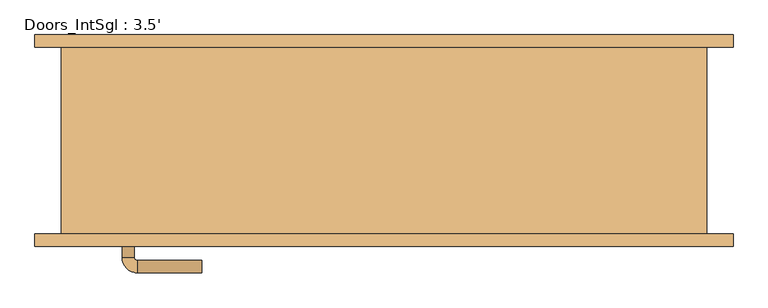
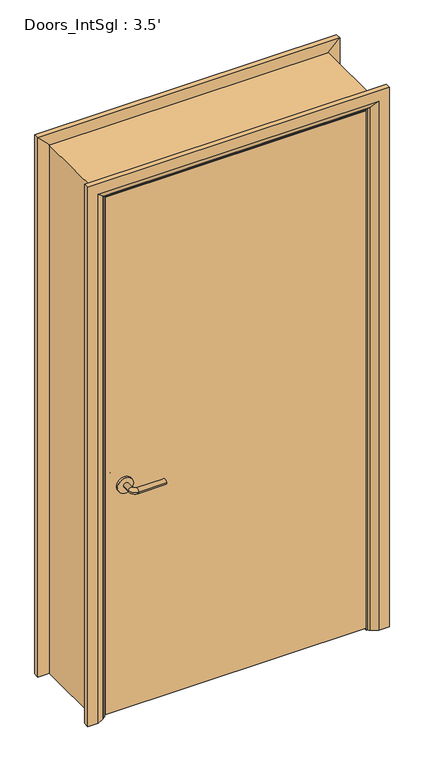
"""IFC4 building model written with IfcOpenShell, lengths in millimetres: door geometry, Doors_IntSgl : 3.5'."""

from ifc_helpers import new_model, si_unit, point, frame, frame_2d, origin, place, context, project, spatial, polyline, circle_curve, ellipse_curve, trimmed, segment, composite_curve, outline, extrude, faceted_brep, source, transform, mapped, element, save
from ifc_brep_helpers import plane_surface, cylinder_surface, revolved_surface, advanced_brep


def doors_intsgl_3_5_f2e8c556(model_context):
    return source(origin(), model_context, "Body", "SolidModel", [
        advanced_brep(
        [(-426.4, -106.4, 900.0), (-406.4, -106.4, 900.0), (-426.4, -76.4, 900.0), (-406.4, -76.4, 900.0), (-401.4, -71.4, 900.0), (-401.4, -51.4, 900.0), (-296.4, -51.4, 900.0), (-296.4, -71.4, 900.0)],
        [
            (0, 1, circle_curve(frame((-416.4, -106.4, 900.0), z_axis=(0.0, -1.0, 0.0), x_axis=(1.0, 0.0, 0.0)), 10.0)),
            (1, 0, circle_curve(frame((-416.4, -106.4, 900.0), z_axis=(0.0, -1.0, 0.0), x_axis=(1.0, 0.0, 0.0)), 10.0)),
            (0, 2),
            (2, 3, circle_curve(frame((-416.4, -76.4, 900.0), z_axis=(0.0, -1.0, 0.0), x_axis=(1.0, 0.0, 0.0)), 10.0)),
            (3, 1),
            (3, 2, circle_curve(frame((-416.4, -76.4, 900.0), z_axis=(0.0, -1.0, 0.0), x_axis=(1.0, 0.0, 0.0)), 10.0)),
            (4, 3, circle_curve(frame((-401.4, -76.4, 900.0), z_axis=(0.0, 0.0, 1.0), x_axis=(-1.0, 0.0, 0.0)), 5.0)),
            (2, 5, circle_curve(frame((-401.4, -76.4, 900.0), z_axis=(0.0, 0.0, -1.0), x_axis=(-1.0, 0.0, 0.0)), 25.0)),
            (5, 4, circle_curve(frame((-401.4, -61.4, 900.0), z_axis=(-1.0, 0.0, 0.0), x_axis=(0.0, -1.0, 0.0)), 10.0)),
            (4, 5, circle_curve(frame((-401.4, -61.4, 900.0), z_axis=(-1.0, 0.0, 0.0), x_axis=(0.0, -1.0, 0.0)), 10.0)),
            (6, 7, circle_curve(frame((-296.4, -61.4, 900.0), z_axis=(1.0, 0.0, 0.0), x_axis=(0.0, -1.0, 0.0)), 10.0)),
            (7, 6, circle_curve(frame((-296.4, -61.4, 900.0), z_axis=(1.0, 0.0, 0.0), x_axis=(0.0, -1.0, 0.0)), 10.0)),
            (5, 6),
            (7, 4),
        ],
        [
            plane_surface(frame((-416.4, -106.4, 900.0), z_axis=(0.0, -1.0, 0.0), x_axis=(0.0, 0.0, 1.0))),
            cylinder_surface(frame((-416.4, -106.4, 900.0), z_axis=(0.0, -1.0, 0.0), x_axis=(1.0, 0.0, 0.0)), 10.0),
            revolved_surface(trimmed(ellipse_curve(frame((-416.4, -76.4, 900.0), z_axis=(0.0, -1.0, 0.0), x_axis=(1.0, 0.0, 0.0)), 10.0, 10.0), [point((-426.4, -76.4, 900.0))], [point((-406.4, -76.4, 900.0))], True, "CARTESIAN"), (-401.4, -76.4, 900.0), (0.0, 0.0, -1.0)),
            revolved_surface(trimmed(ellipse_curve(frame((-416.4, -76.4, 900.0), z_axis=(0.0, -1.0, 0.0), x_axis=(1.0, 0.0, 0.0)), 10.0, 10.0), [point((-406.4, -76.4, 900.0))], [point((-426.4, -76.4, 900.0))], True, "CARTESIAN"), (-401.4, -76.4, 900.0), (0.0, 0.0, -1.0)),
            plane_surface(frame((-296.4, -61.4, 900.0), z_axis=(1.0, 0.0, 0.0), x_axis=(0.0, 0.0, 1.0))),
            cylinder_surface(frame((-401.4, -61.4, 900.0), z_axis=(-1.0, 0.0, 0.0), x_axis=(0.0, -1.0, 0.0)), 10.0),
        ],
        [
            (0, [[1, 2]]),
            (1, [[-1, 3, 4, 5]]),
            (1, [[-2, -5, 6, -3]]),
            (2, [[7, -4, 8, 9]]),
            (3, [[-8, -6, -7, 10]]),
            (4, [[11, 12]]),
            (5, [[-9, 13, -12, 14]]),
            (5, [[-10, -14, -11, -13]]),
        ],
    ),
        extrude(outline(composite_curve([segment(trimmed(circle_curve(frame_2d((900.0, -418.9)), 30.0), [point((900.0, -448.9))], [point((900.0, -388.9))], False, "CARTESIAN"), True, "CONTINUOUS"), segment(trimmed(circle_curve(frame_2d((900.0, -418.9)), 30.0), [point((900.0, -388.9))], [point((900.0, -448.9))], False, "CARTESIAN"), True, "CONTINUOUS")], self_intersect=False)), frame((0.0, -114.4, 0.0), z_axis=(0.0, 1.0, 0.0), x_axis=(0.0, 0.0, 1.0)), (0.0, 0.0, 1.0), 8.0),
        advanced_brep(
        [(-426.4, -160.4, 900.0), (-406.4, -160.4, 900.0), (-406.4, -190.4, 900.0), (-426.4, -190.4, 900.0), (-401.4, -195.4, 900.0), (-401.4, -215.4, 900.0), (-296.4, -215.4, 900.0), (-296.4, -195.4, 900.0)],
        [
            (0, 1, circle_curve(frame((-416.4, -160.4, 900.0), z_axis=(0.0, 1.0, 0.0), x_axis=(1.0, 0.0, 0.0)), 10.0)),
            (1, 0, circle_curve(frame((-416.4, -160.4, 900.0), z_axis=(0.0, 1.0, 0.0), x_axis=(1.0, 0.0, 0.0)), 10.0)),
            (1, 2),
            (2, 3, circle_curve(frame((-416.4, -190.4, 900.0), z_axis=(0.0, 1.0, 0.0), x_axis=(1.0, 0.0, 0.0)), 10.0)),
            (3, 0),
            (3, 2, circle_curve(frame((-416.4, -190.4, 900.0), z_axis=(0.0, 1.0, 0.0), x_axis=(1.0, 0.0, 0.0)), 10.0)),
            (4, 5, circle_curve(frame((-401.4, -205.4, 900.0), z_axis=(-1.0, 0.0, 0.0), x_axis=(0.0, 1.0, 0.0)), 10.0)),
            (5, 3, circle_curve(frame((-401.4, -190.4, 900.0), z_axis=(0.0, 0.0, -1.0), x_axis=(-1.0, 0.0, 0.0)), 25.0)),
            (2, 4, circle_curve(frame((-401.4, -190.4, 900.0), z_axis=(0.0, 0.0, 1.0), x_axis=(-1.0, 0.0, 0.0)), 5.0)),
            (5, 4, circle_curve(frame((-401.4, -205.4, 900.0), z_axis=(-1.0, 0.0, 0.0), x_axis=(0.0, 1.0, 0.0)), 10.0)),
            (6, 7, circle_curve(frame((-296.4, -205.4, 900.0), z_axis=(1.0, 0.0, 0.0), x_axis=(0.0, 1.0, 0.0)), 10.0)),
            (7, 6, circle_curve(frame((-296.4, -205.4, 900.0), z_axis=(1.0, 0.0, 0.0), x_axis=(0.0, 1.0, 0.0)), 10.0)),
            (4, 7),
            (6, 5),
        ],
        [
            plane_surface(frame((-416.4, -160.4, 900.0), z_axis=(0.0, 1.0, 0.0), x_axis=(0.0, 0.0, 1.0))),
            cylinder_surface(frame((-416.4, -160.4, 900.0), z_axis=(0.0, 1.0, 0.0), x_axis=(1.0, 0.0, 0.0)), 10.0),
            revolved_surface(trimmed(ellipse_curve(frame((-416.4, -190.4, 900.0), z_axis=(0.0, -1.0, 0.0), x_axis=(1.0, 0.0, 0.0)), 10.0, 10.0), [point((-426.4, -190.4, 900.0))], [point((-406.4, -190.4, 900.0))], True, "CARTESIAN"), (-401.4, -190.4, 900.0), (0.0, 0.0, -1.0)),
            revolved_surface(trimmed(ellipse_curve(frame((-416.4, -190.4, 900.0), z_axis=(0.0, -1.0, 0.0), x_axis=(1.0, 0.0, 0.0)), 10.0, 10.0), [point((-406.4, -190.4, 900.0))], [point((-426.4, -190.4, 900.0))], True, "CARTESIAN"), (-401.4, -190.4, 900.0), (0.0, 0.0, -1.0)),
            plane_surface(frame((-296.4, -205.4, 900.0), z_axis=(1.0, 0.0, 0.0), x_axis=(0.0, 0.0, 1.0))),
            cylinder_surface(frame((-401.4, -205.4, 900.0), z_axis=(-1.0, 0.0, 0.0), x_axis=(0.0, 1.0, 0.0)), 10.0),
        ],
        [
            (0, [[1, 2]]),
            (1, [[3, 4, 5, -2]]),
            (1, [[-5, 6, -3, -1]]),
            (2, [[7, 8, -4, 9]]),
            (3, [[10, -9, -6, -8]]),
            (4, [[11, 12]]),
            (5, [[13, -11, 14, -7]]),
            (5, [[-14, -12, -13, -10]]),
        ],
    ),
        extrude(outline(composite_curve([segment(trimmed(circle_curve(frame_2d((900.0, -418.9)), 30.0), [point((900.0, -448.9))], [point((900.0, -388.9))], False, "CARTESIAN"), True, "CONTINUOUS"), segment(trimmed(circle_curve(frame_2d((900.0, -418.9)), 30.0), [point((900.0, -388.9))], [point((900.0, -448.9))], False, "CARTESIAN"), True, "CONTINUOUS")], self_intersect=False)), frame((0.0, -160.4, 0.0), z_axis=(0.0, 1.0, 0.0), x_axis=(0.0, 0.0, 1.0)), (0.0, 0.0, 1.0), 8.0),
        extrude(outline(polyline([(491.4, -114.4), (491.4, -152.4), (-491.4, -152.4), (-491.4, -114.4), (491.4, -114.4)])), frame((0.0, 0.0, 8.0), z_axis=(0.0, 0.0, 1.0), x_axis=(1.0, 0.0, 0.0)), (0.0, 0.0, 1.0), 2060.0),
        advanced_brep(
        [(568.4, -172.4, 0.0), (528.4, -172.4, 0.0), (502.4, -158.4, 0.0), (498.4, -152.4, 0.0), (568.4, -152.4, 0.0), (568.4, -152.4, 2145.0), (568.4, -172.4, 2145.0), (498.4, -152.4, 2075.0), (-498.4, -152.4, 2075.0), (-498.4, -152.4, 0.0), (-568.4, -152.4, 0.0), (-568.4, -152.4, 2145.0), (502.4, -158.4, 2079.0), (528.4, -172.4, 2105.0), (-568.4, -172.4, 2145.0), (-568.4, -172.4, 0.0), (-528.4, -172.4, 0.0), (-528.4, -172.4, 2105.0), (-502.4, -158.4, 0.0), (-502.4, -158.4, 2079.0)],
        [
            (0, 1),
            (1, 2),
            (2, 3, circle_curve(frame((506.4, -151.4, 0.0), z_axis=(0.0, 0.0, -1.0), x_axis=(1.0, 0.0, 0.0)), 8.0622577)),
            (3, 4),
            (4, 0),
            (4, 5),
            (5, 6),
            (6, 0),
            (3, 7),
            (7, 8),
            (8, 9),
            (9, 10),
            (10, 11),
            (11, 5),
            (2, 12),
            (12, 7, ellipse_curve(frame((506.4, -151.4, 2083.0), z_axis=(0.7071067811865475, 0.0, -0.7071067811865475), x_axis=(-0.7071067811865474, 0.0, -0.7071067811865476)), 11.4017543, 8.0622577)),
            (1, 13),
            (13, 12),
            (6, 14),
            (14, 15),
            (15, 16),
            (16, 17),
            (17, 13),
            (10, 15),
            (14, 11),
            (9, 18, circle_curve(frame((-506.4, -151.4, 0.0), z_axis=(0.0, 0.0, -1.0), x_axis=(-1.0, 0.0, 0.0)), 8.0622577)),
            (18, 16),
            (19, 18),
            (8, 19, ellipse_curve(frame((-506.4, -151.4, 2083.0), z_axis=(-0.7071067811865475, 0.0, -0.7071067811865475), x_axis=(-0.7071067811865474, 0.0, 0.7071067811865476)), 11.4017543, 8.0622577)),
            (19, 17),
            (12, 19),
        ],
        [
            plane_surface(frame((498.4, -152.4, 0.0), z_axis=(0.0, 0.0, -1.0), x_axis=(0.0, 1.0, 0.0))),
            plane_surface(frame((568.4, -172.4, 0.0), z_axis=(1.0, 0.0, 0.0), x_axis=(0.0, 0.0, 1.0))),
            plane_surface(frame((568.4, -152.4, 0.0), z_axis=(0.0, 1.0, 0.0), x_axis=(0.0, 0.0, 1.0))),
            cylinder_surface(frame((506.4, -151.4, 0.0), z_axis=(0.0, 0.0, -1.0), x_axis=(1.0, 0.0, 0.0)), 8.0622577),
            plane_surface(frame((502.4, -158.4, 0.0), z_axis=(-0.4740998230350126, -0.880471099922178, 0.0), x_axis=(0.0, 0.0, 1.0))),
            plane_surface(frame((528.4, -172.4, 0.0), z_axis=(0.0, -1.0, 0.0), x_axis=(0.0, 0.0, 1.0))),
            plane_surface(frame((-568.4, -172.4, 2145.0), z_axis=(-1.0, 0.0, 0.0), x_axis=(0.0, 0.0, -1.0))),
            plane_surface(frame((-498.4, -152.4, 0.0), z_axis=(0.0, 0.0, -1.0), x_axis=(0.0, 1.0, 0.0))),
            cylinder_surface(frame((-506.4, -151.4, 2075.0), z_axis=(0.0, 0.0, 1.0), x_axis=(-1.0, 0.0, 0.0)), 8.0622577),
            plane_surface(frame((-502.4, -158.4, 2079.0), z_axis=(0.47409982303501835, -0.8804710999221749, 0.0), x_axis=(0.0, 0.0, -1.0))),
            plane_surface(frame((568.4, -172.4, 2145.0), z_axis=(0.0, 0.0, 1.0), x_axis=(-1.0, 0.0, 0.0))),
            cylinder_surface(frame((498.4, -151.4, 2083.0), z_axis=(1.0, 0.0, 0.0), x_axis=(0.0, 0.0, 1.0)), 8.0622577),
            plane_surface(frame((502.4, -158.4, 2079.0), z_axis=(0.0, -0.8804710999221764, -0.47409982303501547), x_axis=(-1.0, 0.0, 0.0))),
        ],
        [
            (0, [[1, 2, 3, 4, 5]]),
            (1, [[6, 7, 8, -5]]),
            (2, [[9, 10, 11, 12, 13, 14, -6, -4]]),
            (3, [[15, 16, -9, -3]]),
            (4, [[17, 18, -15, -2]]),
            (5, [[-8, 19, 20, 21, 22, 23, -17, -1]]),
            (6, [[-13, 24, -20, 25]]),
            (7, [[-24, -12, 26, 27, -21]]),
            (8, [[28, -26, -11, 29]]),
            (9, [[-22, -27, -28, 30]]),
            (10, [[-14, -25, -19, -7]]),
            (11, [[31, -29, -10, -16]]),
            (12, [[-23, -30, -31, -18]]),
        ],
    ),
        extrude(outline(polyline([(0.0, -474.4), (2051.0, -474.4), (2051.0, 474.4), (0.0, 474.4), (0.0, 493.4), (2070.0, 493.4), (2070.0, -493.4), (0.0, -493.4), (0.0, -474.4)])), frame((0.0, -112.4, 0.0), z_axis=(0.0, 1.0, 0.0), x_axis=(0.0, 0.0, 1.0)), (0.0, 0.0, 1.0), 32.0),
        advanced_brep(
        [(-568.4, 172.4, 0.0), (-528.4, 172.4, 0.0), (-502.4, 158.4, 0.0), (-498.4, 152.4, 0.0), (-568.4, 152.4, 0.0), (-568.4, 152.4, 2145.0), (-568.4, 172.4, 2145.0), (-498.4, 152.4, 2075.0), (-502.4, 158.4, 2079.0), (-528.4, 172.4, 2105.0), (568.4, 172.4, 0.0), (568.4, 152.4, 0.0), (498.4, 152.4, 0.0), (502.4, 158.4, 0.0), (528.4, 172.4, 0.0), (568.4, 172.4, 2145.0), (528.4, 172.4, 2105.0), (502.4, 158.4, 2079.0), (498.4, 152.4, 2075.0), (568.4, 152.4, 2145.0)],
        [
            (0, 1),
            (1, 2),
            (2, 3, circle_curve(frame((-506.4, 151.4, 0.0), z_axis=(0.0, 0.0, -1.0), x_axis=(-1.0, 0.0, 0.0)), 8.0622577)),
            (3, 4),
            (4, 0),
            (4, 5),
            (5, 6),
            (6, 0),
            (3, 7),
            (7, 5),
            (2, 8),
            (8, 7, ellipse_curve(frame((-506.4, 151.4, 2083.0), z_axis=(-0.7071067811865475, 0.0, -0.7071067811865475), x_axis=(0.7071067811865474, 0.0, -0.7071067811865476)), 11.4017543, 8.0622577)),
            (1, 9),
            (9, 8),
            (6, 9),
            (10, 11),
            (11, 12),
            (12, 13, circle_curve(frame((506.4, 151.4, 0.0), z_axis=(0.0, 0.0, -1.0), x_axis=(1.0, 0.0, 0.0)), 8.0622577)),
            (13, 14),
            (14, 10),
            (15, 10),
            (14, 16),
            (16, 15),
            (13, 17),
            (17, 16),
            (12, 18),
            (18, 17, ellipse_curve(frame((506.4, 151.4, 2083.0), z_axis=(0.7071067811865475, 0.0, -0.7071067811865475), x_axis=(0.7071067811865474, 0.0, 0.7071067811865476)), 11.4017543, 8.0622577)),
            (11, 19),
            (19, 18),
            (15, 19),
            (5, 19),
            (15, 6),
            (7, 18),
            (8, 17),
            (9, 16),
        ],
        [
            plane_surface(frame((-498.4, 225.2010989, 0.0), z_axis=(0.0, 0.0, -1.0), x_axis=(1.0, 0.0, 0.0))),
            plane_surface(frame((-568.4, 172.4, 0.0), z_axis=(-1.0, 0.0, 0.0), x_axis=(0.0, 0.0, 1.0))),
            plane_surface(frame((-568.4, 152.4, 0.0), z_axis=(0.0, -1.0, 0.0), x_axis=(0.0, 0.0, 1.0))),
            cylinder_surface(frame((-506.4, 151.4, 0.0), z_axis=(0.0, 0.0, -1.0), x_axis=(-1.0, 0.0, 0.0)), 8.0622577),
            plane_surface(frame((-502.4, 158.4, 0.0), z_axis=(0.4740998230350183, 0.8804710999221749, 0.0), x_axis=(0.0, 0.0, 1.0))),
            plane_surface(frame((-528.4, 172.4, 0.0), z_axis=(0.0, 1.0, 0.0), x_axis=(0.0, 0.0, 1.0))),
            plane_surface(frame((498.4, 225.2010989, 0.0), z_axis=(0.0, 0.0, -1.0), x_axis=(-1.0, 0.0, 0.0))),
            plane_surface(frame((528.4, 172.4, 2105.0), z_axis=(0.0, 1.0, 0.0), x_axis=(0.0, 0.0, -1.0))),
            plane_surface(frame((502.4, 158.4, 2079.0), z_axis=(-0.4740998230350183, 0.8804710999221749, 0.0), x_axis=(0.0, 0.0, -1.0))),
            cylinder_surface(frame((506.4, 151.4, 2075.0), z_axis=(0.0, 0.0, 1.0), x_axis=(1.0, 0.0, 0.0)), 8.0622577),
            plane_surface(frame((568.4, 152.4, 2145.0), z_axis=(0.0, -1.0, 0.0), x_axis=(0.0, 0.0, -1.0))),
            plane_surface(frame((568.4, 172.4, 2145.0), z_axis=(1.0, 0.0, 0.0), x_axis=(0.0, 0.0, -1.0))),
            plane_surface(frame((-568.4, 172.4, 2145.0), z_axis=(0.0, 0.0, 1.0), x_axis=(1.0, 0.0, 0.0))),
            plane_surface(frame((-568.4, 152.4, 2145.0), z_axis=(0.0, -1.0, 0.0), x_axis=(1.0, 0.0, 0.0))),
            cylinder_surface(frame((-498.4, 151.4, 2083.0), z_axis=(-1.0, 0.0, 0.0), x_axis=(0.0, 0.0, 1.0)), 8.0622577),
            plane_surface(frame((-502.4, 158.4, 2079.0), z_axis=(0.0, 0.8804710999221749, -0.4740998230350183), x_axis=(1.0, 0.0, 0.0))),
            plane_surface(frame((-528.4, 172.4, 2105.0), z_axis=(0.0, 1.0, 0.0), x_axis=(1.0, 0.0, 0.0))),
        ],
        [
            (0, [[1, 2, 3, 4, 5]]),
            (1, [[6, 7, 8, -5]]),
            (2, [[9, 10, -6, -4]]),
            (3, [[11, 12, -9, -3]]),
            (4, [[13, 14, -11, -2]]),
            (5, [[-8, 15, -13, -1]]),
            (6, [[16, 17, 18, 19, 20]]),
            (7, [[21, -20, 22, 23]]),
            (8, [[-22, -19, 24, 25]]),
            (9, [[-24, -18, 26, 27]]),
            (10, [[-26, -17, 28, 29]]),
            (11, [[-28, -16, -21, 30]]),
            (12, [[31, -30, 32, -7]]),
            (13, [[33, -29, -31, -10]]),
            (14, [[34, -27, -33, -12]]),
            (15, [[35, -25, -34, -14]]),
            (16, [[-32, -23, -35, -15]]),
        ],
    ),
        faceted_brep([(-493.4, -152.4, 0.0), (-525.4, -152.4, 0.0), (-525.4, 152.4, 0.0), (-493.4, 152.4, 0.0), (-493.4, 152.4, 2070.0), (-493.4, -152.4, 2070.0), (-525.4, 152.4, 2102.0), (-525.4, -152.4, 2102.0), (493.4, -152.4, 0.0), (493.4, 152.4, 0.0), (525.4, 152.4, 0.0), (525.4, -152.4, 0.0), (493.4, -152.4, 2070.0), (525.4, -152.4, 2102.0), (525.4, 152.4, 2102.0), (493.4, 152.4, 2070.0)], [[[0, 1, 2, 3]], [[3, 4, 5, 0]], [[2, 6, 4, 3]], [[1, 7, 6, 2]], [[0, 5, 7, 1]], [[8, 9, 10, 11]], [[12, 8, 11, 13]], [[13, 11, 10, 14]], [[14, 10, 9, 15]], [[15, 9, 8, 12]], [[4, 15, 12, 5]], [[6, 14, 15, 4]], [[7, 13, 14, 6]], [[5, 12, 13, 7]]]),
    ])


if __name__ == "__main__":
    model = new_model("IFC4")
    model_context = context("Model", 3, world=origin())
    ifc_project = project(units=[si_unit("LENGTHUNIT", "METRE", prefix="MILLI")], contexts=[model_context])
    site = spatial("IfcSite", under=ifc_project)
    building = spatial("IfcBuilding", under=site)
    placement = place(None, origin())
    doors_intsgl_3_5_shape = doors_intsgl_3_5_f2e8c556(model_context)
    element("IfcDoor", 1, ObjectType="Doors_IntSgl : 3.5'", at=placement, inside=building, context=model_context, shape_type="MappedRepresentation", body=[
        mapped(doors_intsgl_3_5_shape, transform((0.0, 0.0, 0.0), x_axis=(1.0, 0.0, 0.0), y_axis=(0.0, 1.0, 0.0), z_axis=(0.0, 0.0, 1.0))),
    ])
    save(model, "model.ifc")

# Revit data of these elements
# Type "Doors_IntSgl : 3.5'"
#   Type Mark = "51"
#   Type Comments = "Internal Single"
#   Operation = "SingleSwingRight"
#   Manufacturer = "Revit"
#   Keynote = "L20"
#   Description = "Internal Single Door"
#   Analytic Construction = "Metal"
#   UnderCut = 0.026247 ft
#   Tolerance = 0.006562 ft
#   Thickness = 0.124672 ft
#   Thermal Resistance (R) = 0.270117 (m²·K)/W
#   Structural Tolerance = 0.026247 ft
#   StopDepth = 0.104987 ft
#   Stop Thickness = 0.062336 ft
#   Rough Width = 3.5 ft
#   Rough Height = 6.922572 ft
#   Height to Top Lock Rail = 3.28084 ft
#   Heat Transfer Coefficient (U) = 3.7021 W/(m²·K)
#   Handle Z Distance = 2.952756 ft
#   Handle X Distance = 0.246063 ft
#   Frame Thickness = 0.104987 ft
#   Door Panel Width = 3.224409 ft
#   Door Panel Thickness = 0.124672 ft
#   Door Panel Offset = 0.0 ft
#   Height = 6.922572 ft
#   Width = 3.5 ft
#   Door Panel Height = 6.75853 ft
#   Architrave Setback = 0.016404 ft
#   Vis - Ironmongery = yes
#   Material Ironmongery = Door - Handle
#   Material Frame = Door - Frame/Mullion (1)
#   Material Door = Door - Panel
#   Material Architrave = Door - Architrave
#   Visual Light Transmittance = 0
#   Solar Heat Gain Coefficient = 0
#   Function = (empty or 0)
#   Wall Closure = (empty or 0)
# Element 1 (IfcDoor, "Doors_IntSgl : 3.5'")
#   Materials on its faces: "Door - Architrave", "Door - Handle", "Door - Frame/Mullion (1)", "Door - Panel"
# Materials
#   "Door - Handle": colour RGB 0 0 0, transparency 0, Keynote = "P21", Cost = 0
#   "Door - Frame/Mullion (1)": class "Wood", colour RGB 212 179 113, transparency 0, Keynote = "L20", Cost = 0
#   "Door - Panel": class "Wood", colour RGB 210 159 95, transparency 0, Keynote = "L20", Cost = 0
#   "Door - Architrave": class "Wood", colour RGB 154 90 5, transparency 0, Keynote = "P20", Cost = 0
